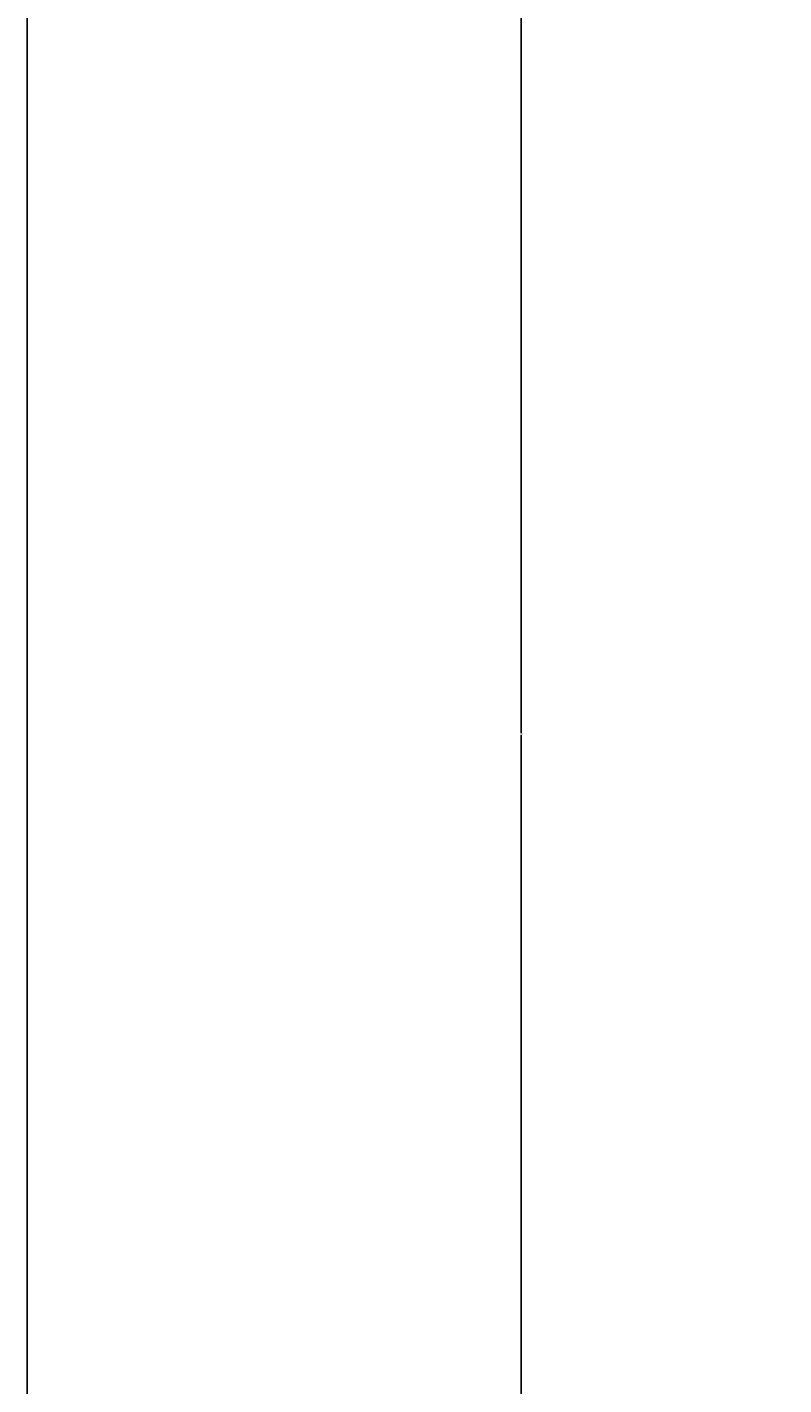
# Model space of a CAD drawing. Units: inches. Extents: x 2168 to 3056, y 1130 to 2629.
# Tile 3 of 42: x 2168 to 2329, y 1789 to 2079. Entities that reach past the tile are written whole.
import ezdxf

# ---------------------------------------------------------------- set-up
doc = ezdxf.new("R2010")
doc.units = ezdxf.units.IN
doc.layers.add('A-ANNO-DIMS', color=2, linetype='Continuous', lineweight=18)
doc.layers.add('A-ANNO-TTLB', color=7, linetype='Continuous', lineweight=25)
doc.styles.get("Standard").update_dxf_attribs({"font": 'arial.ttf'})
doc.dimstyles.get("Standard").update_dxf_attribs({"dimtxt": 0.18, "dimasz": 0.18, "dimexe": 0.18, "dimexo": 0.0625, "dimgap": 0.09, "dimtad": 0, "dimtih": 1, "dimtoh": 1, "dimdec": 4, "dimzin": 0, "dimdsep": 46, "dimtxsty": 'Standard', "dimcen": 0.09, "dimadec": 0, "dimazin": 0, "dimtfac": 1, "dimtdec": 4, "dimtofl": 0, "dimtmove": 0, "dimatfit": 3, "dimfxl": 1, "dimtolj": 1, "dimtzin": 0, "dimarcsym": 0})

# ---------------------------------------------------------------- blocks, each defined once
blk = doc.blocks.new('*D41')
at = {"layer": 'A-ANNO-DIMS', "color": 0, "lineweight": -2, "transparency": 16777216}
for p, q in [((2331.73, 2478.39), (2273.32, 2478.39)), ((2273.5, 2478.21), (2273.5, 1928.07)), ((2273.5, 1377.57), (2273.5, 1927.71)), ((2331.73, 1377.39), (2273.32, 1377.39))]:
    blk.add_line(p, q, dxfattribs=at)
at = {"layer": 'A-ANNO-DIMS', "color": 0, "transparency": 16777216}
for points in [[(2273.47, 2478.21), (2273.53, 2478.21), (2273.5, 2478.39)], [(2273.47, 1377.57), (2273.53, 1377.57), (2273.5, 1377.39)]]:
    blk.add_solid(points, dxfattribs=at)
at = {"layer": 'Defpoints', "color": 0, "transparency": 16777216}
for p in [(2273.5, 2478.39), (2331.8, 2478.39), (2331.8, 1377.39)]:
    blk.add_point(p, dxfattribs=at)
at = {"layer": 'A-ANNO-DIMS', "color": 0, "transparency": 16777216, "insert": (2273.5, 1927.89), "char_height": 0.18, "attachment_point": 5}
blk.add_mtext('\\A1;1101', dxfattribs=at)

msp = doc.modelspace()

# ---------------------------------------------------------------- linework, layer by layer
at = {"layer": 'A-ANNO-TTLB'}
msp.add_lwpolyline([(2168.16, 2629.19), (3055.63, 2629.19), (3055.63, 1130.19), (2168.16, 1130.19)], close=True, dxfattribs=at)

# ---------------------------------------------------------------- dimensions: what is measured, and where the dimension line sits
at = {"layer": 'A-ANNO-DIMS'}
dim = msp.add_linear_dim(base=(2273.5, 2478.39), p1=(2331.8, 1377.39), p2=(2331.8, 2478.39), angle=90, dimstyle='Standard', override={"dimdec": 0, "dimlfac": 1, "dimrnd": 0, "dimzin": 0, "dimdsep": 46, "dimlunit": 2}, dxfattribs=at)
dim.commit()
dim.dimension.update_dxf_attribs({"geometry": '*D41', "text_midpoint": (2273.5, 1927.89)})

doc.saveas('drawing.dxf')
